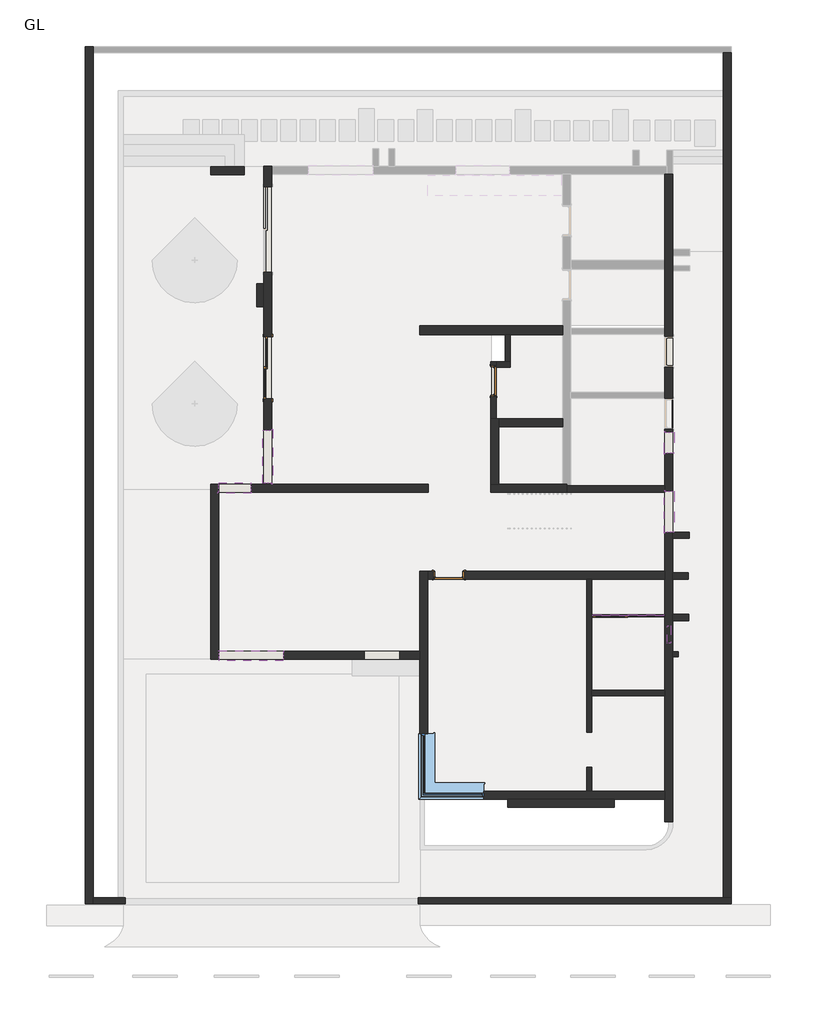
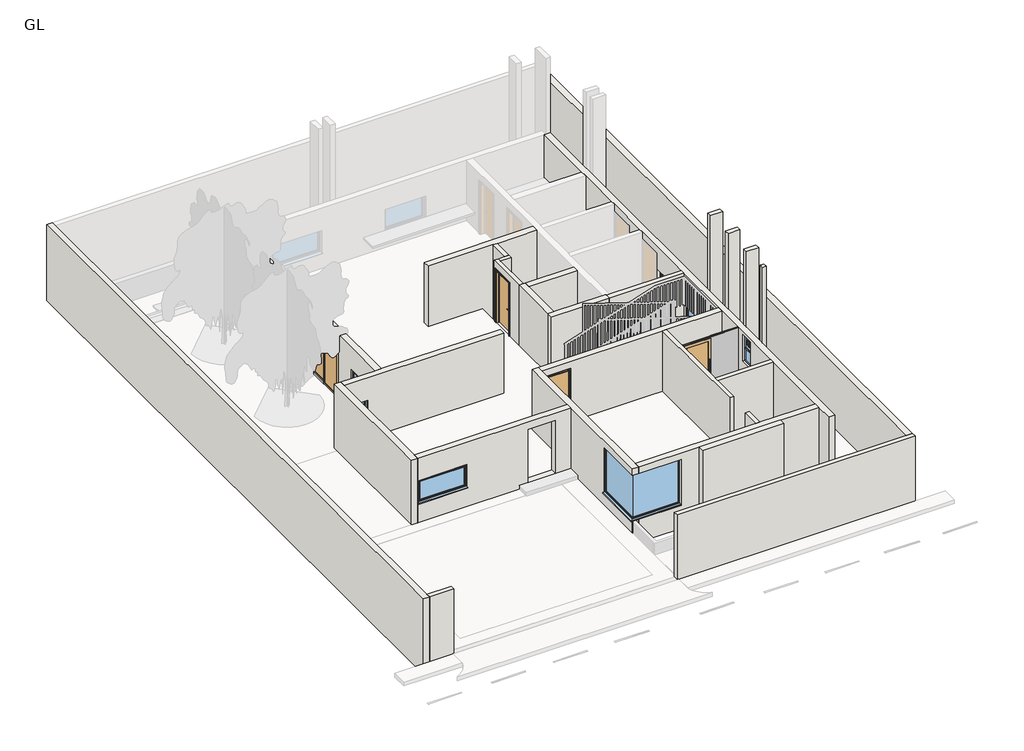
# One storey, part 1 of 6: 30 walls, 7 members, 7 windows, 4 doors, 1 plate.
# Revit data of these elements (continued)
# Type "Windows_Sgl_Plain : 3'" (continued)
#   Wall Closure = (empty or 0)
# Type "Windows_Sgl_Plain : 3'10\""
#   Type Mark = "68"
#   Operation = "SinglePanel"
#   Construction Type Id = "SGL"
#   Manufacturer = "Revit"
#   Keynote = "L10"
#   Analytic Construction = "Large single-glazed windows"
#   Wrap Layers (Ext) from Ext = 0' - 4.03543"
#   Wrap Layers (Int) from Ext = 0' - 6.98819"
#   Window Board Projection = 0' - 0.98425"
#   Window Board Extension = 0' - 0.98425"
#   Visual Light Transmittance = 0.9
#   Solar Heat Gain Coefficient = 0.86
#   Rough Width = 3' - 10"
#   Rough Height = 2' - 11.82677"
#   Height = 2' - 11.82677"
#   Width = 3' - 10"
#   Heat Transfer Coefficient (U) = 5.5617 W/(m²·K)
#   Glazing Thickness = 0' - 0.94488"
#   FrameOffset - External = 0' - 1.9685"
#   Frame Depth = 0' - 2.55906"
#   Default Head Height = 6' - 11.07087"
#   Cill Depth = 0' - 3.44488"
#   Cavity Closer Width = 0' - 1.9685"
#   Cavity Closer Offset from Ext = 0' - 4.03543"
#   Cavity Closer Depth = 0' - 3.34646"
#   Vis - Cavity Closers = yes
#   Define Thermal Properties by = 1
#   Material Trim = Window Frame
#   Material Glass = Glass
#   Material Frame = Window Frame
#   Wall Closure = (empty or 0)
# Type "Windows_Sgl_Plain : 5'"
#   Type Mark = "67"
#   Operation = "SinglePanel"
#   Construction Type Id = "SGL"
#   Manufacturer = "Revit"
#   Keynote = "L10"
#   Analytic Construction = "Large single-glazed windows"
#   Wrap Layers (Ext) from Ext = 0' - 4.03543"
#   Wrap Layers (Int) from Ext = 0' - 6.98819"
#   Window Board Projection = 0' - 0.98425"
#   Window Board Extension = 0' - 0.98425"
#   Visual Light Transmittance = 0.9
#   Solar Heat Gain Coefficient = 0.86
#   Rough Width = 5' - 0"
#   Rough Height = 2' - 11.82677"
#   Height = 2' - 11.82677"
#   Width = 5' - 0"
#   Heat Transfer Coefficient (U) = 5.5617 W/(m²·K)
#   Glazing Thickness = 0' - 0.94488"
#   FrameOffset - External = 0' - 1.9685"
#   Frame Depth = 0' - 2.55906"
#   Default Head Height = 6' - 11.07087"
#   Cill Depth = 0' - 3.44488"
#   Cavity Closer Width = 0' - 1.9685"
#   Cavity Closer Offset from Ext = 0' - 4.03543"
#   Cavity Closer Depth = 0' - 3.34646"
#   Vis - Cavity Closers = yes
#   Define Thermal Properties by = 1
#   Material Trim = Window Frame
#   Material Glass = Glass
#   Material Frame = Window Frame
#   Wall Closure = (empty or 0)
# Type "Windows_Sgl_Plain : 6'"
#   Type Mark = "69"
#   Operation = "SinglePanel"
#   Construction Type Id = "SGL"
#   Manufacturer = "Revit"
#   Keynote = "L10"
#   Analytic Construction = "Large single-glazed windows"
#   Wrap Layers (Ext) from Ext = 0' - 4.03543"
#   Wrap Layers (Int) from Ext = 0' - 6.98819"
#   Window Board Projection = 0' - 0.98425"
#   Window Board Extension = 0' - 0.98425"
#   Visual Light Transmittance = 0.9
#   Solar Heat Gain Coefficient = 0.86
#   Rough Width = 6' - 0"
#   Rough Height = 2' - 11.82677"
#   Height = 2' - 11.82677"
#   Width = 6' - 0"
#   Heat Transfer Coefficient (U) = 5.5617 W/(m²·K)
#   Glazing Thickness = 0' - 0.94488"
#   FrameOffset - External = 0' - 1.9685"
#   Frame Depth = 0' - 2.55906"
#   Default Head Height = 6' - 11.07087"
#   Cill Depth = 0' - 3.44488"
#   Cavity Closer Width = 0' - 1.9685"
#   Cavity Closer Offset from Ext = 0' - 4.03543"
#   Cavity Closer Depth = 0' - 3.34646"
#   Vis - Cavity Closers = yes
#   Define Thermal Properties by = 1
#   Material Trim = Window Frame
#   Material Glass = Glass
#   Material Frame = Window Frame
#   Wall Closure = (empty or 0)
# Element 1 (IfcDoor, "5'10\"")
#   Phase Created = New Construction
#   Materials on its faces: "Puerta - Panel", "Cristal"
# Elements 2, 3 (IfcDoor, "Doors_IntSgl : 2'11\"")
#   Phase Created = New Construction
#   Materials on its faces: "Door - Architrave", "Door - Handle", "Door - Frame/Mullion (1)", "Door - Panel"
# Element 4 (IfcDoor, "Doors_Sgl_Glass_1 : Glass_Panel-12mm_Thickness")
#   Phase Created = New Construction
#   Materials on its faces: "Metal - Aluminum", "Glass"
# Elements 5, 6, 7, 8, 9, 10, 11 (IfcMember, "Rectangular Mullion : 30mm_Square")
#   Phase Created = New Construction
#   Materials on its faces: "Aluminium"
# Element 12 (IfcPlate, "System Panel : Glazed")
#   Phase Created = New Construction
#   Materials on its faces: "Glass"
# Elements 13, 14, 15, 16, 17, 18 (IfcWall, "6\" WALL")
#   Top Offset = 0' - 0"
#   Base Offset = 0' - 0"
#   wall height = 9' - 10.11024"
#   Phase Created = New Construction
#   Base Constraint = GL
#   Top Constraint = FFL
#   Materials on its faces: "Brick, Common"
# Element 19 (IfcWall, "6\" WALL")
#   Top Offset = 0' - 0"
#   Base Offset = 0' - 0"
#   wall height = 19' - 8.22047"
#   Phase Created = New Construction
#   Base Constraint = GL
#   Top Constraint = SFL
#   Materials on its faces: "Brick, Common"
# Elements 20, 21, 22 (IfcWall, "7\" WALL")
#   Top Offset = 0' - 0"
#   Base Offset = 0' - 0"
#   wall height = 9' - 10.11024"
#   Phase Created = New Construction
#   Base Constraint = GL
#   Top Constraint = FFL
#   Materials on its faces: "Brick, Common"
# Elements 23, 24, 25 (IfcWall, "7\" WALL")
#   Top Offset = 0' - 0"
#   Base Offset = 0' - 0"
#   wall height = 19' - 8.22047"
#   Phase Created = New Construction
#   Base Constraint = GL
#   Top Constraint = SFL
#   Materials on its faces: "Brick, Common"
# Element 26 (IfcWall, "8\" WALL")
#   Top Offset = 0' - 0"
#   Base Offset = 0' - 0"
#   wall height = 9' - 10.11024"
#   Phase Created = New Construction
#   Base Constraint = GL
#   Top Constraint = FFL
#   Materials on its faces: "Brick, Common"
# Elements 27, 28, 29, 30, 31, 32, 33, 34, 35, 36, 37, 38, 39, 40, 41 (IfcWall, "9\" INNER WALL")
#   Top Offset = 0' - 0"
#   Base Offset = 0' - 0"
#   wall height = 9' - 10.11024"
#   Phase Created = New Construction
#   Base Constraint = GL
#   Top Constraint = FFL
#   Materials on its faces: "Brick, Common"
# Element 42 (IfcWall, "9\" INNER WALL 2")
#   Top Offset = 0' - 0"
#   Base Offset = 0' - 0"
#   wall height = 9' - 10.11024"
#   Phase Created = New Construction
#   Base Constraint = GL
#   Top Constraint = FFL
#   Materials on its faces: "Brick, Common"
# Element 43 (IfcWindow, "Bathroom-Window-with-Vent_Fan : B")
#   Mark = "2"
#   Phase Created = New Construction
#   Materials on its faces: "Plastic", "Aluminium", "Glass"
# Element 44 (IfcWindow, "Windows_Corner : 1829x1829mm 2")
#   Mark = "1"
#   Wall/Void Thickness = 1' - 3.74803"
#   Phase Created = New Construction
#   Materials on its faces: "Window Frame", "Glass"
# Element 45 (IfcWindow, "Windows_Sgl_Plain : 2'")
#   Mark = "20"
#   Phase Created = New Construction
#   Materials on its faces: "Window Frame", "Glass"
# Element 46 (IfcWindow, "Windows_Sgl_Plain : 3'")
#   Mark = "24"
#   Phase Created = New Construction
#   Materials on its faces: "Window Frame", "Glass"
# Element 47 (IfcWindow, "Windows_Sgl_Plain : 3'10\"")
#   Mark = "19"
#   Phase Created = New Construction
#   Materials on its faces: "Window Frame", "Glass"
# Element 48 (IfcWindow, "Windows_Sgl_Plain : 5'")
#   Mark = "23"
#   Phase Created = New Construction
#   Materials on its faces: "Window Frame", "Glass"
# Element 49 (IfcWindow, "Windows_Sgl_Plain : 6'")
#   Mark = "25"
#   Phase Created = New Construction
#   Materials on its faces: "Window Frame", "Glass"
# Materials
#   "Puerta - Panel": class "Madera", colour RGB 210 159 95, transparency 0
#   "Door - Handle": colour RGB 0 0 0, transparency 0, Keynote = "P21", Cost = 0
#   "Door - Frame/Mullion (1)": class "Wood", colour RGB 212 179 113, transparency 0, Keynote = "L20", Cost = 0
#   "Door - Panel": class "Wood", colour RGB 210 159 95, transparency 0, Keynote = "L20", Cost = 0
#   "Door - Architrave": class "Wood", colour RGB 154 90 5, transparency 0, Keynote = "P20", Cost = 0
#   "Metal - Aluminum": class "Metal", colour RGB 247 247 247, transparency 0
#   "Glass": class "Glass", colour RGB 0 128 192, transparency 0.9, Description = "Soda Lime Glass", Cost = 0
#   "Brick, Common": class "Masonry", colour RGB 170 100 105, transparency 0, Description = "Common brick", Cost = 0
#   "Aluminium": class "Metal", colour RGB 247 247 247, transparency 0, Description = "Aluminium 6061", Cost = 0
#   "Plastic": class "Plastic", colour RGB 0 0 0, transparency 0, Description = "Generic Plastic", Cost = 0
#   "Window Frame": colour RGB 249 249 249, transparency 0, Keynote = "L10", Cost = 0
#   "Cristal": class "Vidrio", colour RGB 0 0 255, transparency 0.75
